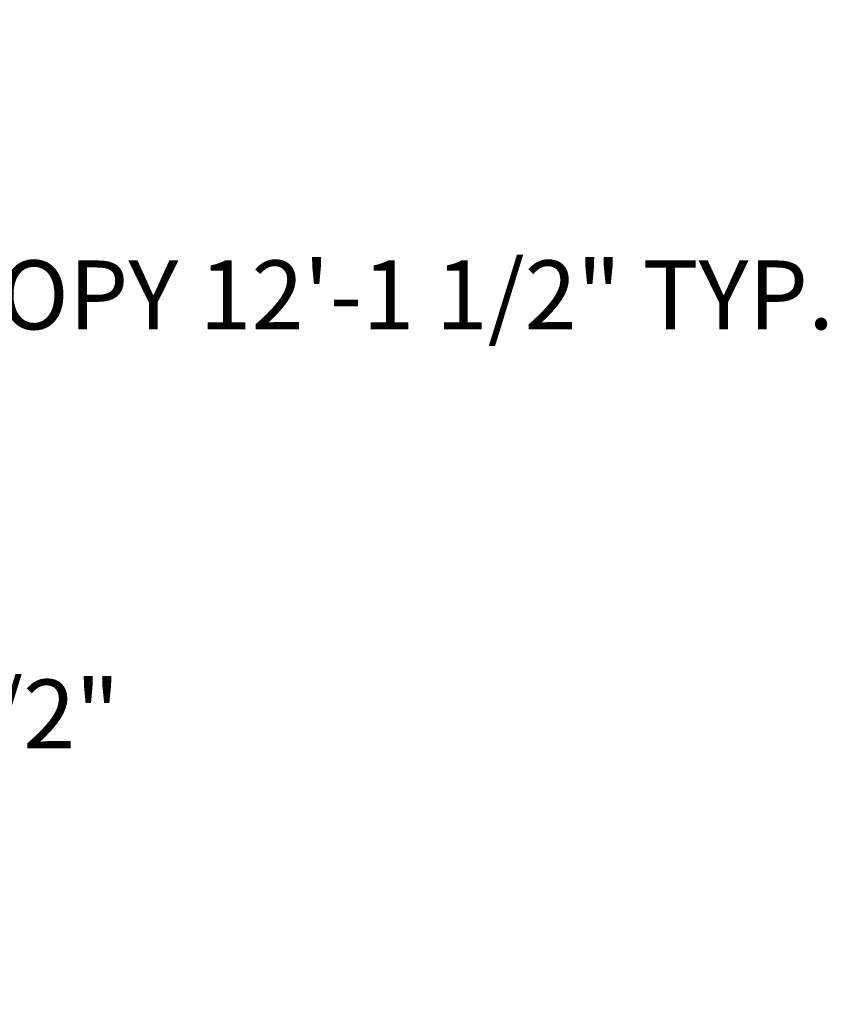
# Model space of a CAD drawing. Units: inches. Extents: x 28 to 3832, y 2 to 1709.
# Tile 7 of 7: x 3536 to 3832, y 1021 to 1381. Entities that reach past the tile are written whole.
import ezdxf

# ---------------------------------------------------------------- set-up
doc = ezdxf.new("R2010")
doc.units = ezdxf.units.IN
doc.header["$MEASUREMENT"] = 0
doc.layers.add('A-ANNO-DIMS', color=2, linetype='Continuous', lineweight=18)
doc.styles.get("Standard").update_dxf_attribs({"font": 'arial.ttf'})
doc.dimstyles.get("Standard").update_dxf_attribs({"dimtxt": 25.18, "dimasz": 20.18, "dimexe": 0.18, "dimexo": 0.0625, "dimgap": 0.09, "dimtad": 0, "dimtih": 1, "dimtoh": 1, "dimdec": 0, "dimzin": 0, "dimdsep": 46, "dimlunit": 3, "dimtxsty": 'Standard', "dimcen": 0.09, "dimadec": 0, "dimazin": 0, "dimtfac": 1, "dimtdec": 0, "dimtofl": 0, "dimtmove": 0, "dimatfit": 3, "dimfxl": 1, "dimtolj": 1, "dimtzin": 0, "dimarcsym": 0})

# ---------------------------------------------------------------- blocks, each defined once
blk = doc.blocks.new('*D45')
at = {"layer": 'A-ANNO-DIMS', "color": 0, "lineweight": -2, "transparency": 16777216}
for p, q in [((3166.51, 1302.58), (3166.51, 1280.67)), ((3311.78, 1302.58), (3311.78, 1280.67)), ((3186.69, 1280.85), (3291.6, 1280.85)), ((3311.78, 1280.85), (3331.96, 1280.85))]:
    blk.add_line(p, q, dxfattribs=at)
at = {"layer": 'A-ANNO-DIMS', "color": 0, "transparency": 16777216}
for points in [[(3186.69, 1284.21), (3186.69, 1277.49), (3166.51, 1280.85)], [(3291.6, 1284.21), (3291.6, 1277.49), (3311.78, 1280.85)]]:
    blk.add_solid(points, dxfattribs=at)
at = {"layer": 'Defpoints', "color": 0, "transparency": 16777216}
for p in [(3166.51, 1302.64), (3311.78, 1302.64), (3311.78, 1280.85)]:
    blk.add_point(p, dxfattribs=at)
at = {"layer": 'A-ANNO-DIMS', "color": 0, "transparency": 16777216, "insert": (3590.91, 1280.85), "char_height": 25.18, "attachment_point": 5}
blk.add_mtext('\\A1;ENTRY CANOPY 12\'-1 1/2" TYP.', dxfattribs=at)
blk = doc.blocks.new('*D57')
at = {"layer": 'A-ANNO-DIMS', "color": 0, "lineweight": -2, "transparency": 16777216}
for p, q in [((3422.07, 1107.41), (3422.07, 1127.59)), ((3422.07, 1127.59), (3442.25, 1127.59)), ((3341.88, 1087.23), (3422.25, 1087.23)), ((3396.68, 1061.8), (3422.25, 1061.8)), ((3422.07, 1041.62), (3422.07, 1021.44))]:
    blk.add_line(p, q, dxfattribs=at)
at = {"layer": 'A-ANNO-DIMS', "color": 0, "transparency": 16777216}
for points in [[(3418.71, 1107.41), (3425.43, 1107.41), (3422.07, 1087.23)], [(3418.71, 1041.62), (3425.43, 1041.62), (3422.07, 1061.8)]]:
    blk.add_solid(points, dxfattribs=at)
at = {"layer": 'Defpoints', "color": 0, "transparency": 16777216}
for p in [(3341.81, 1087.23), (3422.07, 1087.23), (3396.62, 1061.8)]:
    blk.add_point(p, dxfattribs=at)
at = {"layer": 'A-ANNO-DIMS', "color": 0, "transparency": 16777216, "insert": (3505.36, 1127.59), "char_height": 25.18, "attachment_point": 5}
blk.add_mtext('\\A1;2\'-1 1/2"', dxfattribs=at)

msp = doc.modelspace()

# ---------------------------------------------------------------- dimensions: what is measured, and where the dimension line sits
at = {"layer": 'A-ANNO-DIMS'}
dim = msp.add_linear_dim(base=(3311.78, 1280.85), p1=(3166.51, 1302.64), p2=(3311.78, 1302.64), text='ENTRY CANOPY <> TYP.', dimstyle='Standard', override={"dimdec": 1, "dimlfac": 1, "dimrnd": 0, "dimzin": 1, "dimdsep": 46, "dimlunit": 4, "dimfrac": 2}, dxfattribs=at)
dim.commit()
dim.dimension.update_dxf_attribs({"geometry": '*D45', "text_midpoint": (3590.91, 1280.85)})
dim = msp.add_linear_dim(base=(3422.07, 1087.23), p1=(3396.62, 1061.8), p2=(3341.81, 1087.23), angle=90, dimstyle='Standard', override={"dimdec": 1, "dimlfac": 1, "dimrnd": 0, "dimzin": 1, "dimdsep": 46, "dimlunit": 4, "dimfrac": 2}, dxfattribs=at)
dim.commit()
dim.dimension.update_dxf_attribs({"geometry": '*D57', "text_midpoint": (3505.36, 1127.59)})

doc.saveas('drawing.dxf')
